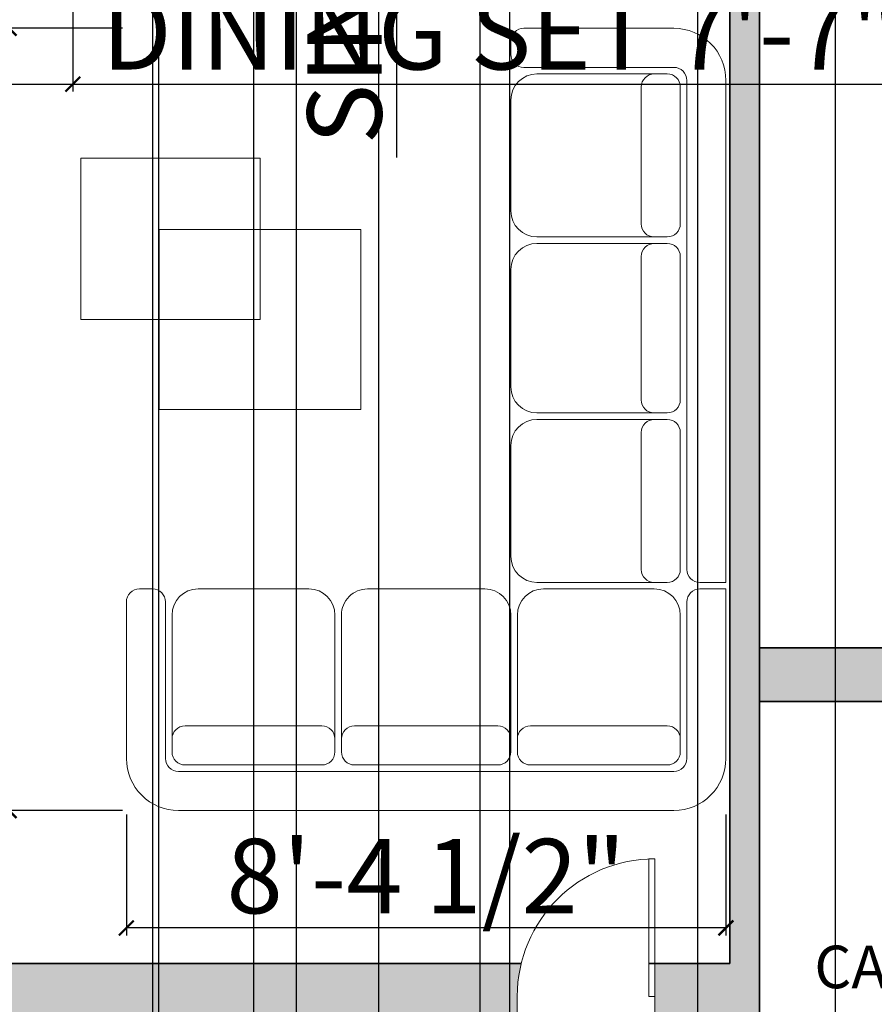
# Model space of a CAD drawing. Units: inches. Extents: x 1763 to 2368, y 1500 to 2097.
# Tile 4 of 24: x 1936 to 2079, y 1628 to 1794. Entities that reach past the tile are written whole.
import ezdxf

# ---------------------------------------------------------------- set-up
doc = ezdxf.new("R2010")
doc.units = ezdxf.units.IN
for name, color, linetype, lineweight in [('A-ANNO-DIMS', 2, 'Continuous', 18), ('A-AREA-IDEN', 7, 'Continuous', 18), ('A-DOOR', 4, 'Continuous', 18), ('A-FURN', 8, 'Continuous', 18), ('A-WALL', 7, 'Continuous', 35), ('A-WALL-PATT', 7, 'Continuous', 13)]:
    doc.layers.add(name, color=color, linetype=linetype, lineweight=lineweight)
doc.styles.get("Standard").update_dxf_attribs({"font": 'arial.ttf'})
doc.dimstyles.new('ISO-25', dxfattribs={"dimtxt": 12.5, "dimasz": 2.5, "dimexe": 1.25, "dimexo": 0.625, "dimtad": 1, "dimdec": 0, "dimlunit": 4, "dimtxsty": 'Standard', "dimblk": 'ARCHTICK', "dimcen": 2.5, "dimclrd": 3, "dimclrt": 4, "dimadec": 0, "dimazin": 0, "dimtfac": 1, "dimtdec": 0, "dimtmove": 0, "dimatfit": 3, "dimfxl": 1, "dimarcsym": 0})

# ---------------------------------------------------------------- blocks, each defined once
blk = doc.blocks.new('A$C2AFA021D')
for p, q in [((0.8, 2.3), (0.2, 2.3)), ((0.85, 2.2), (0.85, 2.25)), ((0.2, 2.15), (0.8, 2.15)), ((0.225, 2.125), (0.275, 2.125)), ((0.75, 2.125), (0.275, 2.125)), ((0, 2.1), (0, 0.2)), ((0.15, 0.2), (0.15, 2.1)), ((0.175, 1.55), (0.175, 2.075)), ((0.325, 2.075), (0.325, 1.55)), ((0.85, 1.6), (0.85, 2.025)), ((0.275, 1.5), (0.225, 1.5)), ((0.225, 1.475), (0.275, 1.475)), ((0.275, 1.5), (0.75, 1.5)), ((0.75, 1.475), (0.275, 1.475)), ((0.175, 0.875), (0.175, 1.425)), ((0.325, 1.425), (0.325, 0.875)), ((0.85, 0.925), (0.85, 1.375)), ((0.275, 0.825), (0.225, 0.825)), ((0.225, 0.8), (0.275, 0.8)), ((0.275, 0.825), (0.75, 0.825)), ((0.75, 0.8), (0.275, 0.8)), ((0.975, 0.825), (1.4, 0.825)), ((1.625, 0.825), (2.075, 0.825)), ((2.3, 0.825), (2.725, 0.825)), ((2.9, 0.825), (2.95, 0.825)), ((2.85, 0.2), (2.85, 0.775)), ((3, 0.775), (3, 0.2)), ((0.175, 0.225), (0.175, 0.75)), ((0.325, 0.75), (0.325, 0.225)), ((0.875, 0.275), (0.875, 0.725)), ((1.5, 0.725), (1.5, 0.275)), ((1.525, 0.275), (1.525, 0.725)), ((2.175, 0.725), (2.175, 0.275)), ((2.2, 0.275), (2.2, 0.725)), ((2.825, 0.725), (2.825, 0.275)), ((0.85, 0.275), (0.85, 0.7)), ((1.45, 0.325), (0.925, 0.325)), ((2.125, 0.325), (1.575, 0.325)), ((2.775, 0.325), (2.25, 0.325)), ((0.875, 0.275), (0.875, 0.225)), ((1.5, 0.225), (1.5, 0.275)), ((1.525, 0.275), (1.525, 0.225)), ((2.175, 0.225), (2.175, 0.275)), ((2.2, 0.275), (2.2, 0.225)), ((2.825, 0.225), (2.825, 0.275)), ((0.275, 0.175), (0.225, 0.175)), ((0.275, 0.175), (0.75, 0.175)), ((0.925, 0.175), (1.45, 0.175)), ((1.575, 0.175), (2.125, 0.175)), ((2.25, 0.175), (2.775, 0.175)), ((0.8, 0.15), (0.2, 0.15)), ((0.925, 0.15), (2.8, 0.15)), ((0.85, 0), (0.85, 0.1)), ((0.875, 0.1), (0.875, 0)), ((0.2, 0), (0.85, 0)), ((2.8, 0), (0.875, 0))]:
    blk.add_line(p, q)
for centre, radius, start, end in [((0.2, 2.1), 0.2, 90, 180), ((0.8, 2.25), 0.05, 0, 90), ((0.8, 2.2), 0.05, 270, 0), ((0.2, 2.1), 0.05, 90, 180), ((0.225, 2.075), 0.05, 90, 180), ((0.275, 2.075), 0.05, 0, 90), ((0.75, 2.025), 0.1, 0, 90), ((0.75, 1.6), 0.1, 270, 0), ((0.225, 1.55), 0.05, 180, 270), ((0.275, 1.55), 0.05, 270, 0), ((0.225, 1.425), 0.05, 90, 180), ((0.275, 1.425), 0.05, 0, 90), ((0.75, 1.375), 0.1, 360, 90), ((0.75, 0.925), 0.1, 270, 0), ((0.225, 0.875), 0.05, 180, 270), ((0.275, 0.875), 0.05, 270, 0), ((0.225, 0.75), 0.05, 90, 180), ((0.275, 0.75), 0.05, 0, 90), ((0.75, 0.7), 0.1, 0, 90), ((0.975, 0.725), 0.1, 90, 180), ((1.4, 0.725), 0.1, 0, 90), ((1.625, 0.725), 0.1, 90, 180), ((2.075, 0.725), 0.1, 0, 90), ((2.3, 0.725), 0.1, 90, 180), ((2.725, 0.725), 0.1, 0, 90), ((2.9, 0.775), 0.05, 90, 180), ((2.95, 0.775), 0.05, 0, 90), ((0.925, 0.275), 0.05, 90, 180), ((1.45, 0.275), 0.05, 360, 90), ((1.575, 0.275), 0.05, 90, 180), ((2.125, 0.275), 0.05, 360, 90), ((2.25, 0.275), 0.05, 90, 180), ((2.775, 0.275), 0.05, 360, 90), ((0.75, 0.275), 0.1, 270, 0), ((0.2, 0.2), 0.2, 180, 270), ((0.2, 0.2), 0.05, 180, 270), ((0.225, 0.225), 0.05, 180, 270), ((0.275, 0.225), 0.05, 270, 0), ((0.925, 0.225), 0.05, 180, 270), ((1.45, 0.225), 0.05, 270, 0), ((1.575, 0.225), 0.05, 180, 270), ((2.125, 0.225), 0.05, 270, 0), ((2.25, 0.225), 0.05, 180, 270), ((2.775, 0.225), 0.05, 270, 0), ((2.8, 0.2), 0.2, 270, 0), ((2.8, 0.2), 0.05, 270, 0), ((0.8, 0.1), 0.05, 0, 90), ((0.925, 0.1), 0.05, 90, 180)]:
    blk.add_arc(centre, radius, start, end)
blk = doc.blocks.new('*U3')
for p, q in [((0, 0), (0, -6)), ((40, 0), (40, -6))]:
    blk.add_line(p, q)
blk.add_lwpolyline([(0, 0), (0, 40), (1.75, 40), (1.75, 0)], close=True)
blk.add_arc((0, 0), 40, 0, 90)
blk = doc.blocks.new('_ArchTick')
at = {"color": 0, "linetype": 'ByBlock', "const_width": 0.15}
blk.add_lwpolyline([(-0.5, -0.5), (0.5, 0.5)], dxfattribs=at)
blk = doc.blocks.new('*D25')
at = {"layer": 'A-ANNO-DIMS', "color": 3, "lineweight": -2, "transparency": 16777216}
for p, q in [((1934.01, 1792.31), (1934.01, 1981.61)), ((1934.01, 1660.94), (1934.01, 1792.31))]:
    blk.add_line(p, q, dxfattribs=at)
at = {"layer": 'A-ANNO-DIMS', "color": 0, "lineweight": -2, "transparency": 16777216}
for p, q in [((1953.09, 1792.31), (1932.76, 1792.31)), ((1953.09, 1660.94), (1932.76, 1660.94))]:
    blk.add_line(p, q, dxfattribs=at)
at = {"layer": 'Defpoints', "color": 0, "transparency": 16777216}
for p in [(1934.01, 1792.31), (1953.72, 1792.31), (1953.72, 1660.94)]:
    blk.add_point(p, dxfattribs=at)
at = {"layer": 'A-ANNO-DIMS', "color": 3, "lineweight": -2, "transparency": 16777216, "xscale": 2.5, "yscale": 2.5, "zscale": 2.5}
for p, rotation in [((1934.01, 1792.31), 90), ((1934.01, 1660.94), 270)]:
    blk.add_blockref('_ArchTick', p, dxfattribs=dict(at, rotation=rotation))
at = {"layer": 'A-ANNO-DIMS', "color": 4, "transparency": 16777216, "insert": (1926.92, 1888.21), "char_height": 12.5, "attachment_point": 5, "rotation": 90}
blk.add_mtext('SECTIONAL 10\'-11 1/2"', dxfattribs=at)
blk = doc.blocks.new('*D26')
at = {"layer": 'A-ANNO-DIMS', "color": 0, "lineweight": -2, "transparency": 16777216}
for p, q in [((1953.72, 1660.31), (1953.72, 1639.98)), ((2054.44, 1660.31), (2054.44, 1639.98))]:
    blk.add_line(p, q, dxfattribs=at)
at = {"layer": 'A-ANNO-DIMS', "color": 3, "lineweight": -2, "transparency": 16777216}
blk.add_line((2054.44, 1641.23), (1953.72, 1641.23), dxfattribs=at)
at = {"layer": 'Defpoints', "color": 0, "transparency": 16777216}
for p in [(1953.72, 1660.94), (2054.44, 1660.94), (1953.72, 1641.23)]:
    blk.add_point(p, dxfattribs=at)
at = {"layer": 'A-ANNO-DIMS', "color": 3, "lineweight": -2, "transparency": 16777216, "xscale": 2.5, "yscale": 2.5, "zscale": 2.5, "rotation": 180}
blk.add_blockref('_ArchTick', (1953.72, 1641.23), dxfattribs=at)
at = {"layer": 'A-ANNO-DIMS', "color": 3, "lineweight": -2, "transparency": 16777216, "xscale": 2.5, "yscale": 2.5, "zscale": 2.5}
blk.add_blockref('_ArchTick', (2054.44, 1641.23), dxfattribs=at)
at = {"layer": 'A-ANNO-DIMS', "color": 4, "transparency": 16777216, "insert": (2004.08, 1648.32), "char_height": 12.5, "attachment_point": 5}
blk.add_mtext('8\'-4 1/2"', dxfattribs=at)
blk = doc.blocks.new('*D27')
at = {"layer": 'A-ANNO-DIMS', "color": 0, "lineweight": -2, "transparency": 16777216}
for p, q in [((1853.71, 1795.96), (1853.71, 1781.68)), ((1944.71, 1795.96), (1944.71, 1781.68))]:
    blk.add_line(p, q, dxfattribs=at)
at = {"layer": 'A-ANNO-DIMS', "color": 3, "lineweight": -2, "transparency": 16777216}
for p, q in [((1853.71, 1782.93), (1944.71, 1782.93)), ((1944.71, 1782.93), (2085.85, 1782.93))]:
    blk.add_line(p, q, dxfattribs=at)
at = {"layer": 'Defpoints', "color": 0, "transparency": 16777216}
for p in [(1853.71, 1796.58), (1944.71, 1796.58), (1944.71, 1782.93)]:
    blk.add_point(p, dxfattribs=at)
at = {"layer": 'A-ANNO-DIMS', "color": 3, "lineweight": -2, "transparency": 16777216, "xscale": 2.5, "yscale": 2.5, "zscale": 2.5, "rotation": 180}
blk.add_blockref('_ArchTick', (1853.71, 1782.93), dxfattribs=at)
at = {"layer": 'A-ANNO-DIMS', "color": 3, "lineweight": -2, "transparency": 16777216, "xscale": 2.5, "yscale": 2.5, "zscale": 2.5}
blk.add_blockref('_ArchTick', (1944.71, 1782.93), dxfattribs=at)
at = {"layer": 'A-ANNO-DIMS', "color": 4, "transparency": 16777216, "insert": (2016.53, 1790.02), "char_height": 12.5, "attachment_point": 5}
blk.add_mtext('DINING SET 7\'-7"', dxfattribs=at)
blk = doc.blocks.new('*D33')
at = {"layer": 'A-ANNO-DIMS', "color": 0, "lineweight": -2, "transparency": 16777216}
for p, q in [((2001.02, 1913.28), (1997.82, 1913.28)), ((2001.02, 1896.11), (1997.82, 1896.11))]:
    blk.add_line(p, q, dxfattribs=at)
at = {"layer": 'A-ANNO-DIMS', "color": 3, "lineweight": -2, "transparency": 16777216}
for p, q in [((1999.07, 1913.28), (1999.07, 1896.11)), ((1999.07, 1896.11), (1999.07, 1770.61))]:
    blk.add_line(p, q, dxfattribs=at)
at = {"layer": 'Defpoints', "color": 0, "transparency": 16777216}
for p in [(2001.64, 1913.28), (1999.07, 1896.11), (2001.64, 1896.11)]:
    blk.add_point(p, dxfattribs=at)
at = {"layer": 'A-ANNO-DIMS', "color": 3, "lineweight": -2, "transparency": 16777216, "xscale": 2.5, "yscale": 2.5, "zscale": 2.5}
for p, rotation in [((1999.07, 1913.28), 90), ((1999.07, 1896.11), 270)]:
    blk.add_blockref('_ArchTick', p, dxfattribs=dict(at, rotation=rotation))
at = {"layer": 'A-ANNO-DIMS', "color": 4, "transparency": 16777216, "insert": (1991.98, 1832.11), "char_height": 12.5, "attachment_point": 5, "rotation": 90}
blk.add_mtext('SINK 1\'-5" TYP.', dxfattribs=at)
blk = doc.blocks.new('*D58')
at = {"layer": 'A-ANNO-DIMS', "color": 0, "lineweight": -2, "transparency": 16777216}
for p, q in [((1871.68, 1635.9), (1871.68, 2072.02)), ((1927.07, 1635.9), (1927.07, 2072.02))]:
    blk.add_line(p, q, dxfattribs=at)
at = {"layer": 'A-ANNO-DIMS', "color": 3, "lineweight": -2, "transparency": 16777216}
for p, q in [((1871.68, 2070.77), (1927.07, 2070.77)), ((1927.07, 2070.77), (1993.68, 2070.77))]:
    blk.add_line(p, q, dxfattribs=at)
at = {"layer": 'Defpoints', "color": 0, "transparency": 16777216}
for p in [(1927.07, 2070.77), (1871.68, 1635.27), (1927.07, 1635.27)]:
    blk.add_point(p, dxfattribs=at)
at = {"layer": 'A-ANNO-DIMS', "color": 3, "lineweight": -2, "transparency": 16777216, "xscale": 2.5, "yscale": 2.5, "zscale": 2.5, "rotation": 180}
blk.add_blockref('_ArchTick', (1871.68, 2070.77), dxfattribs=at)
at = {"layer": 'A-ANNO-DIMS', "color": 3, "lineweight": -2, "transparency": 16777216, "xscale": 2.5, "yscale": 2.5, "zscale": 2.5}
blk.add_blockref('_ArchTick', (1927.07, 2070.77), dxfattribs=at)
at = {"layer": 'A-ANNO-DIMS', "color": 4, "transparency": 16777216, "insert": (1961.63, 2077.86), "char_height": 12.5, "attachment_point": 5}
blk.add_mtext('4\'-7 1/2"', dxfattribs=at)
blk = doc.blocks.new('*D60')
at = {"layer": 'A-ANNO-DIMS', "color": 0, "lineweight": -2, "transparency": 16777216}
for p, q in [((2060.09, 1678.65), (2060.09, 1509.91)), ((2100.58, 1678.65), (2100.58, 1509.91))]:
    blk.add_line(p, q, dxfattribs=at)
at = {"layer": 'A-ANNO-DIMS', "color": 3, "lineweight": -2, "transparency": 16777216}
for p, q in [((2060.09, 1511.16), (2100.58, 1511.16)), ((2100.58, 1511.16), (2166.67, 1511.16))]:
    blk.add_line(p, q, dxfattribs=at)
at = {"layer": 'Defpoints', "color": 0, "transparency": 16777216}
for p in [(2060.09, 1679.27), (2100.58, 1679.27), (2100.58, 1511.16)]:
    blk.add_point(p, dxfattribs=at)
at = {"layer": 'A-ANNO-DIMS', "color": 3, "lineweight": -2, "transparency": 16777216, "xscale": 2.5, "yscale": 2.5, "zscale": 2.5, "rotation": 180}
blk.add_blockref('_ArchTick', (2060.09, 1511.16), dxfattribs=at)
at = {"layer": 'A-ANNO-DIMS', "color": 3, "lineweight": -2, "transparency": 16777216, "xscale": 2.5, "yscale": 2.5, "zscale": 2.5}
blk.add_blockref('_ArchTick', (2100.58, 1511.16), dxfattribs=at)
at = {"layer": 'A-ANNO-DIMS', "color": 4, "transparency": 16777216, "insert": (2134.88, 1518.25), "char_height": 12.5, "attachment_point": 5}
blk.add_mtext('3\'-4 1/2"', dxfattribs=at)
blk = doc.blocks.new('*D68')
at = {"layer": 'A-ANNO-DIMS', "color": 0, "lineweight": -2, "transparency": 16777216}
for p, q in [((1895.59, 1879.65), (1895.59, 1509.91)), ((1932.01, 1879.65), (1932.01, 1509.91))]:
    blk.add_line(p, q, dxfattribs=at)
at = {"layer": 'A-ANNO-DIMS', "color": 3, "lineweight": -2, "transparency": 16777216}
for p, q in [((1895.59, 1511.16), (1932.01, 1511.16)), ((1932.01, 1511.16), (1998.11, 1511.16))]:
    blk.add_line(p, q, dxfattribs=at)
at = {"layer": 'Defpoints', "color": 0, "transparency": 16777216}
for p in [(1895.59, 1880.27), (1932.01, 1880.27), (1932.01, 1511.16)]:
    blk.add_point(p, dxfattribs=at)
at = {"layer": 'A-ANNO-DIMS', "color": 3, "lineweight": -2, "transparency": 16777216, "xscale": 2.5, "yscale": 2.5, "zscale": 2.5, "rotation": 180}
blk.add_blockref('_ArchTick', (1895.59, 1511.16), dxfattribs=at)
at = {"layer": 'A-ANNO-DIMS', "color": 3, "lineweight": -2, "transparency": 16777216, "xscale": 2.5, "yscale": 2.5, "zscale": 2.5}
blk.add_blockref('_ArchTick', (1932.01, 1511.16), dxfattribs=at)
at = {"layer": 'A-ANNO-DIMS', "color": 4, "transparency": 16777216, "insert": (1966.31, 1518.25), "char_height": 12.5, "attachment_point": 5}
blk.add_mtext('3\'-0 1/2"', dxfattribs=at)
blk = doc.blocks.new('*D69')
at = {"layer": 'A-ANNO-DIMS', "color": 0, "lineweight": -2, "transparency": 16777216}
for p, q in [((1838.09, 1879.65), (1838.09, 1509.91)), ((1895.59, 1879.65), (1895.59, 1509.91))]:
    blk.add_line(p, q, dxfattribs=at)
at = {"layer": 'A-ANNO-DIMS', "color": 3, "lineweight": -2, "transparency": 16777216}
for p, q in [((1838.09, 1511.16), (1895.59, 1511.16)), ((1895.59, 1511.16), (1962.2, 1511.16))]:
    blk.add_line(p, q, dxfattribs=at)
at = {"layer": 'Defpoints', "color": 0, "transparency": 16777216}
for p in [(1838.09, 1880.27), (1895.59, 1880.27), (1895.59, 1511.16)]:
    blk.add_point(p, dxfattribs=at)
at = {"layer": 'A-ANNO-DIMS', "color": 3, "lineweight": -2, "transparency": 16777216, "xscale": 2.5, "yscale": 2.5, "zscale": 2.5, "rotation": 180}
blk.add_blockref('_ArchTick', (1838.09, 1511.16), dxfattribs=at)
at = {"layer": 'A-ANNO-DIMS', "color": 3, "lineweight": -2, "transparency": 16777216, "xscale": 2.5, "yscale": 2.5, "zscale": 2.5}
blk.add_blockref('_ArchTick', (1895.59, 1511.16), dxfattribs=at)
at = {"layer": 'A-ANNO-DIMS', "color": 4, "transparency": 16777216, "insert": (1930.15, 1518.24), "char_height": 12.5, "attachment_point": 5}
blk.add_mtext('4\'-9 1/2"', dxfattribs=at)
blk = doc.blocks.new('*D70')
at = {"layer": 'A-ANNO-DIMS', "color": 0, "lineweight": -2, "transparency": 16777216}
for p, q in [((1959.13, 1879.65), (1959.13, 1509.91)), ((1982.23, 1879.65), (1982.23, 1509.91))]:
    blk.add_line(p, q, dxfattribs=at)
at = {"layer": 'A-ANNO-DIMS', "color": 3, "lineweight": -2, "transparency": 16777216}
for p, q in [((1959.13, 1511.16), (1982.23, 1511.16)), ((1982.23, 1511.16), (2027.75, 1511.16))]:
    blk.add_line(p, q, dxfattribs=at)
at = {"layer": 'Defpoints', "color": 0, "transparency": 16777216}
for p in [(1959.13, 1880.27), (1982.23, 1880.27), (1982.23, 1511.16)]:
    blk.add_point(p, dxfattribs=at)
at = {"layer": 'A-ANNO-DIMS', "color": 3, "lineweight": -2, "transparency": 16777216, "xscale": 2.5, "yscale": 2.5, "zscale": 2.5, "rotation": 180}
blk.add_blockref('_ArchTick', (1959.13, 1511.16), dxfattribs=at)
at = {"layer": 'A-ANNO-DIMS', "color": 3, "lineweight": -2, "transparency": 16777216, "xscale": 2.5, "yscale": 2.5, "zscale": 2.5}
blk.add_blockref('_ArchTick', (1982.23, 1511.16), dxfattribs=at)
at = {"layer": 'A-ANNO-DIMS', "color": 4, "transparency": 16777216, "insert": (2006.24, 1518.06), "char_height": 12.5, "attachment_point": 5}
blk.add_mtext('1\'-11"', dxfattribs=at)
blk = doc.blocks.new('*D71')
at = {"layer": 'A-ANNO-DIMS', "color": 0, "lineweight": -2, "transparency": 16777216}
for p, q in [((2049.69, 1879.65), (2049.69, 1509.91)), ((2072.78, 1879.65), (2072.78, 1509.91))]:
    blk.add_line(p, q, dxfattribs=at)
at = {"layer": 'A-ANNO-DIMS', "color": 3, "lineweight": -2, "transparency": 16777216}
for p, q in [((2049.69, 1511.16), (2072.78, 1511.16)), ((2072.78, 1511.16), (2118.3, 1511.16))]:
    blk.add_line(p, q, dxfattribs=at)
at = {"layer": 'Defpoints', "color": 0, "transparency": 16777216}
for p in [(2049.69, 1880.27), (2072.78, 1880.27), (2072.78, 1511.16)]:
    blk.add_point(p, dxfattribs=at)
at = {"layer": 'A-ANNO-DIMS', "color": 3, "lineweight": -2, "transparency": 16777216, "xscale": 2.5, "yscale": 2.5, "zscale": 2.5, "rotation": 180}
blk.add_blockref('_ArchTick', (2049.69, 1511.16), dxfattribs=at)
at = {"layer": 'A-ANNO-DIMS', "color": 3, "lineweight": -2, "transparency": 16777216, "xscale": 2.5, "yscale": 2.5, "zscale": 2.5}
blk.add_blockref('_ArchTick', (2072.78, 1511.16), dxfattribs=at)
at = {"layer": 'A-ANNO-DIMS', "color": 4, "transparency": 16777216, "insert": (2096.79, 1518.06), "char_height": 12.5, "attachment_point": 5}
blk.add_mtext('1\'-11"', dxfattribs=at)
blk = doc.blocks.new('*D77')
at = {"layer": 'A-ANNO-DIMS', "color": 0, "lineweight": -2, "transparency": 16777216}
for p, q in [((1975.09, 1972.65), (1975.09, 1509.91)), ((1996.09, 1972.65), (1996.09, 1509.91))]:
    blk.add_line(p, q, dxfattribs=at)
at = {"layer": 'A-ANNO-DIMS', "color": 3, "lineweight": -2, "transparency": 16777216}
for p, q in [((1975.09, 1511.16), (1996.09, 1511.16)), ((1996.09, 1511.16), (2031.89, 1511.16))]:
    blk.add_line(p, q, dxfattribs=at)
at = {"layer": 'Defpoints', "color": 0, "transparency": 16777216}
for p in [(1975.09, 1973.27), (1996.09, 1973.27), (1996.09, 1511.16)]:
    blk.add_point(p, dxfattribs=at)
at = {"layer": 'A-ANNO-DIMS', "color": 3, "lineweight": -2, "transparency": 16777216, "xscale": 2.5, "yscale": 2.5, "zscale": 2.5, "rotation": 180}
blk.add_blockref('_ArchTick', (1975.09, 1511.16), dxfattribs=at)
at = {"layer": 'A-ANNO-DIMS', "color": 3, "lineweight": -2, "transparency": 16777216, "xscale": 2.5, "yscale": 2.5, "zscale": 2.5}
blk.add_blockref('_ArchTick', (1996.09, 1511.16), dxfattribs=at)
at = {"layer": 'A-ANNO-DIMS', "color": 4, "transparency": 16777216, "insert": (2015.24, 1518.16), "char_height": 12.5, "attachment_point": 5}
blk.add_mtext('1\'-9"', dxfattribs=at)
blk = doc.blocks.new('*D86')
at = {"layer": 'A-ANNO-DIMS', "color": 0, "lineweight": -2, "transparency": 16777216}
for p, q in [((2013.09, 1884.65), (2013.09, 1509.91)), ((2018.09, 1884.65), (2018.09, 1509.91))]:
    blk.add_line(p, q, dxfattribs=at)
at = {"layer": 'A-ANNO-DIMS', "color": 3, "lineweight": -2, "transparency": 16777216}
for p, q in [((2013.09, 1511.16), (2018.09, 1511.16)), ((2018.09, 1511.16), (2055.07, 1511.16))]:
    blk.add_line(p, q, dxfattribs=at)
at = {"layer": 'Defpoints', "color": 0, "transparency": 16777216}
for p in [(2013.09, 1885.27), (2018.09, 1885.27), (2018.09, 1511.16)]:
    blk.add_point(p, dxfattribs=at)
at = {"layer": 'A-ANNO-DIMS', "color": 3, "lineweight": -2, "transparency": 16777216, "xscale": 2.5, "yscale": 2.5, "zscale": 2.5, "rotation": 180}
blk.add_blockref('_ArchTick', (2013.09, 1511.16), dxfattribs=at)
at = {"layer": 'A-ANNO-DIMS', "color": 3, "lineweight": -2, "transparency": 16777216, "xscale": 2.5, "yscale": 2.5, "zscale": 2.5}
blk.add_blockref('_ArchTick', (2018.09, 1511.16), dxfattribs=at)
at = {"layer": 'A-ANNO-DIMS', "color": 4, "transparency": 16777216, "insert": (2037.83, 1518.16), "char_height": 12.5, "attachment_point": 5}
blk.add_mtext('0\'-5"', dxfattribs=at)
blk = doc.blocks.new('*D87')
at = {"layer": 'A-ANNO-DIMS', "color": 0, "lineweight": -2, "transparency": 16777216}
for p, q in [((1958.09, 1980.65), (1958.09, 1509.91)), ((1975.09, 1980.65), (1975.09, 1509.91))]:
    blk.add_line(p, q, dxfattribs=at)
at = {"layer": 'A-ANNO-DIMS', "color": 3, "lineweight": -2, "transparency": 16777216}
for p, q in [((1958.09, 1511.16), (1975.09, 1511.16)), ((1975.09, 1511.16), (2010.89, 1511.16))]:
    blk.add_line(p, q, dxfattribs=at)
at = {"layer": 'Defpoints', "color": 0, "transparency": 16777216}
for p in [(1958.09, 1981.27), (1975.09, 1981.27), (1975.09, 1511.16)]:
    blk.add_point(p, dxfattribs=at)
at = {"layer": 'A-ANNO-DIMS', "color": 3, "lineweight": -2, "transparency": 16777216, "xscale": 2.5, "yscale": 2.5, "zscale": 2.5, "rotation": 180}
blk.add_blockref('_ArchTick', (1958.09, 1511.16), dxfattribs=at)
at = {"layer": 'A-ANNO-DIMS', "color": 3, "lineweight": -2, "transparency": 16777216, "xscale": 2.5, "yscale": 2.5, "zscale": 2.5}
blk.add_blockref('_ArchTick', (1975.09, 1511.16), dxfattribs=at)
at = {"layer": 'A-ANNO-DIMS', "color": 4, "transparency": 16777216, "insert": (1994.24, 1518.16), "char_height": 12.5, "attachment_point": 5}
blk.add_mtext('1\'-5"', dxfattribs=at)

msp = doc.modelspace()

# ---------------------------------------------------------------- hatches: boundary and pattern name
at = {"layer": 'A-WALL-PATT'}
h = msp.add_hatch(color=256, dxfattribs=at)
h.dxf.hatch_style = 1
h.paths.add_polyline_path([(1838.09, 2034.27), (1838.09, 2043.27), (1829.09, 2043.27), (1829.09, 1953.39), (1838.09, 1953.39)])
h.paths.add_polyline_path([(1838.09, 1913.1), (1829.09, 1913.1), (1829.09, 1862.2), (1838.09, 1862.2)])
h.paths.add_polyline_path([(1838.09, 1825.59), (1829.09, 1825.59), (1829.09, 1738.64), (1838.09, 1738.64)])
h.paths.add_polyline_path([(1895.59, 1885.27), (1838.09, 1885.27), (1838.09, 1880.27), (1895.59, 1880.27)])
h.paths.add_polyline_path([(1857.39, 1784.27), (1838.09, 1784.27), (1838.09, 1779.27), (1857.39, 1779.27)])
h.paths.add_polyline_path([(1958.09, 1981.27), (1971.46, 1981.27), (1971.46, 1986.27), (1968.57, 1986.27), (1958.09, 1986.27), (1953.09, 1986.27), (1927.39, 1986.27), (1927.39, 1981.27), (1953.09, 1981.27), (1953.09, 1885.27), (1932.01, 1885.27), (1932.01, 1880.27), (1959.13, 1880.27), (1959.13, 1883.74), (1959.13, 1885.27), (1958.09, 1885.27)])
h.paths.add_polyline_path([(2018.09, 1981.27), (2031.02, 1981.27), (2031.02, 1986.27), (2018.09, 1986.27), (2013.09, 1986.27), (2001.23, 1986.27), (2001.23, 1981.27), (2013.09, 1981.27), (2013.09, 1885.27), (1982.18, 1885.27, -0.016629), (1982.23, 1883.74), (1982.23, 1880.27), (2049.69, 1880.27), (2049.69, 1883.74, -0.016629), (2049.74, 1885.27), (2018.09, 1885.27)])
h.paths.add_polyline_path([(2083.09, 1981.27), (2120.61, 1981.27), (2120.61, 1986.27), (2083.09, 1986.27), (2078.09, 1986.27), (2063.14, 1986.27), (2063.14, 1981.27), (2078.09, 1981.27), (2078.09, 1885.27), (2072.78, 1885.27), (2072.78, 1883.74), (2072.78, 1880.27), (2078.09, 1880.27), (2078.09, 1866.87), (2081.56, 1866.87, -0.016629), (2083.09, 1866.82)])
h.paths.add_polyline_path([(1871.68, 1635.27), (1838.09, 1635.27), (1838.09, 1626.27), (1871.68, 1626.27)], flags=17)
h.paths.add_polyline_path([(2100.58, 1688.27), (2060.09, 1688.27), (2060.09, 1679.27), (2100.58, 1679.27)], flags=17)
h.paths.add_polyline_path([(2180.09, 1688.27), (2148.74, 1688.27), (2148.74, 1679.27), (2180.09, 1679.27)], flags=17)
h.paths.add_polyline_path([(2189.09, 1746.22), (2180.09, 1746.22), (2180.09, 1743.42), (2180.12, 1743.42), (2180.12, 1726.72), (2180.09, 1572.27), (2034.91, 1572.27), (2034.91, 1565.6), (2034.91, 1563.27), (2189.09, 1563.27)])
h.paths.add_polyline_path([(2060.09, 1802.35, -0.016629), (2058.56, 1802.3), (2055.09, 1802.3), (2055.09, 1635.27), (2042.48, 1635.27), (2042.48, 1629.74), (2042.48, 1626.27), (2055.09, 1626.27), (2055.09, 1599.27), (2040.27, 1599.27), (2040.27, 1590.27), (2060.09, 1590.27)])
h.paths.add_polyline_path([(2019.39, 1629.74, -0.060569), (2020.06, 1635.27), (1995.09, 1635.27), (1990.09, 1635.27), (1927.07, 1635.27), (1927.07, 1626.27), (1990.09, 1626.27), (1990.09, 1590.27), (1995.09, 1590.27), (2005.2, 1590.27), (2005.2, 1599.27), (1995.09, 1599.27), (1995.09, 1626.27), (2019.39, 1626.27)])
edge = h.paths.add_edge_path()
edge.add_line((2180.09, 1837.27), (2167.2, 1837.27))
edge.add_spline(control_points=[(2167.2, 1837.27), (2167.19, 1837.27), (2167.18, 1837.27), (2167.18, 1837.27)], knot_values=[168.955493, 168.955493, 168.955493, 168.955493, 169.065871, 169.065871, 169.065871, 169.065871], degree=3, periodic=0)
edge.add_spline(control_points=[(2167.18, 1837.27), (2166.56, 1837.38), (2166.33, 1846.16), (2165.71, 1846.24)], knot_values=[159.864705, 159.864705, 159.864705, 159.864705, 168.955493, 168.955493, 168.955493, 168.955493], degree=3, periodic=0)
edge.add_line((2167.12, 1837.27), (2163.16, 1837.27))
edge.add_spline(control_points=[(2163.16, 1837.27), (2163.16, 1837.27), (2163.16, 1837.27), (2163.15, 1837.27)], knot_values=[150.537172, 150.537172, 150.537172, 150.537172, 150.553797, 150.553797, 150.553797, 150.553797], degree=3, periodic=0)
edge.add_spline(control_points=[(2163.15, 1837.27), (2162.29, 1837.29), (2161.59, 1846.23), (2160.88, 1846.24)], knot_values=[141.293426, 141.293426, 141.293426, 141.293426, 150.537172, 150.537172, 150.537172, 150.537172], degree=3, periodic=0)
edge.add_line((2163.08, 1837.27), (2158.7, 1837.27))
edge.add_spline(control_points=[(2158.7, 1837.27), (2158.7, 1837.27), (2158.7, 1837.27), (2158.7, 1837.27)], knot_values=[132.033544, 132.033544, 132.033544, 132.033544, 132.049151, 132.049151, 132.049151, 132.049151], degree=3, periodic=0)
edge.add_spline(control_points=[(2158.7, 1837.27), (2157.97, 1837.29), (2157.26, 1846.23), (2156.39, 1846.24)], knot_values=[122.786021, 122.786021, 122.786021, 122.786021, 132.033544, 132.033544, 132.033544, 132.033544], degree=3, periodic=0)
edge.add_line((2158.63, 1837.27), (2153.84, 1837.27))
edge.add_spline(control_points=[(2153.84, 1837.27), (2153.83, 1837.27), (2153.82, 1837.27), (2153.82, 1837.27)], knot_values=[113.451585, 113.451585, 113.451585, 113.451585, 113.562103, 113.562103, 113.562103, 113.562103], degree=3, periodic=0)
edge.add_spline(control_points=[(2153.82, 1837.27), (2153.17, 1837.38), (2152.88, 1846.19), (2152.4, 1846.24)], knot_values=[0, 0, 0, 0, 9.081854, 9.081854, 9.081854, 9.081854], degree=3, periodic=0)
edge.add_line((2153.76, 1837.27), (2150.39, 1837.27))
edge.add_spline(control_points=[(2150.39, 1837.27), (2150.38, 1837.27), (2150.37, 1837.27), (2150.36, 1837.27)], knot_values=[95.069382, 95.069382, 95.069382, 95.069382, 95.17519, 95.17519, 95.17519, 95.17519], degree=3, periodic=0)
edge.add_spline(control_points=[(2150.36, 1837.27), (2149.49, 1837.37), (2148.42, 1846.19), (2147.59, 1846.24)], knot_values=[85.824599, 85.824599, 85.824599, 85.824599, 95.069382, 95.069382, 95.069382, 95.069382], degree=3, periodic=0)
edge.add_line((2150.29, 1837.27), (2145.43, 1837.27))
edge.add_spline(control_points=[(2145.43, 1837.27), (2145.43, 1837.27), (2145.42, 1837.27), (2145.42, 1837.27)], knot_values=[76.505559, 76.505559, 76.505559, 76.505559, 76.547811, 76.547811, 76.547811, 76.547811], degree=3, periodic=0)
edge.add_spline(control_points=[(2145.42, 1837.27), (2144.68, 1837.31), (2143.8, 1846.19), (2142.95, 1846.24)], knot_values=[67.23945, 67.23945, 67.23945, 67.23945, 76.505559, 76.505559, 76.505559, 76.505559], degree=3, periodic=0)
edge.add_line((2145.35, 1837.27), (2134.57, 1837.27))
edge.add_spline(control_points=[(2134.57, 1837.27), (2134.57, 1837.27), (2134.56, 1837.27), (2134.56, 1837.27)], knot_values=[39.001463, 39.001463, 39.001463, 39.001463, 39.045107, 39.045107, 39.045107, 39.045107], degree=3, periodic=0)
edge.add_spline(control_points=[(2134.56, 1837.27), (2133.87, 1837.31), (2133.4, 1845.85), (2132.33, 1846.24)], knot_values=[29.79778, 29.79778, 29.79778, 29.79778, 39.001463, 39.001463, 39.001463, 39.001463], degree=3, periodic=0)
edge.add_line((2134.5, 1837.27), (2128.08, 1837.27))
edge.add_spline(control_points=[(2128.08, 1837.27), (2128.03, 1837.26), (2127.98, 1837.26), (2127.93, 1837.27)], knot_values=[19.482067, 19.482067, 19.482067, 19.482067, 19.869396, 19.869396, 19.869396, 19.869396], degree=3, periodic=0)
edge.add_spline(control_points=[(2125.01, 1846.24), (2126.16, 1844.66), (2126.82, 1837.57), (2127.93, 1837.27)], knot_values=[10.389805, 10.389805, 10.389805, 10.389805, 19.482067, 19.482067, 19.482067, 19.482067], degree=3, periodic=0)
edge.add_line((2127.93, 1837.27), (2083.09, 1837.27))
edge.add_line((2083.09, 1837.27), (2083.09, 1843.77))
edge.add_line((2083.09, 1843.77), (2081.56, 1843.77))
edge.add_line((2081.56, 1843.77), (2078.09, 1843.77))
edge.add_line((2078.09, 1843.77), (2078.09, 1837.27))
edge.add_line((2078.09, 1837.27), (2055.09, 1837.27))
edge.add_line((2055.09, 1837.27), (2055.09, 1825.4))
edge.add_line((2055.09, 1825.4), (2058.56, 1825.4))
edge.add_line((2058.56, 1825.4), (2060.09, 1825.4))
edge.add_line((2060.09, 1825.4), (2060.09, 1832.27))
edge.add_line((2060.09, 1832.27), (2122.44, 1832.27))
edge.add_spline(control_points=[(2122.44, 1832.27), (2122.73, 1832.58), (2123.01, 1832.62), (2123.28, 1832.27)], knot_values=[5.972033, 5.972033, 5.972033, 5.972033, 8.057258, 8.057258, 8.057258, 8.057258], degree=3, periodic=0)
edge.add_line((2123.28, 1832.27), (2137.95, 1832.27))
edge.add_spline(control_points=[(2137.95, 1832.27), (2137.96, 1832.27), (2137.97, 1832.27), (2137.98, 1832.27)], knot_values=[53.926862, 53.926862, 53.926862, 53.926862, 54.030075, 54.030075, 54.030075, 54.030075], degree=3, periodic=0)
edge.add_spline(control_points=[(2139.72, 1825.02), (2139.28, 1825.06), (2138.67, 1832.18), (2137.98, 1832.27)], knot_values=[54.030075, 54.030075, 54.030075, 54.030075, 61.445194, 61.445194, 61.445194, 61.445194], degree=3, periodic=0)
edge.add_line((2138.05, 1832.27), (2140.96, 1832.27))
edge.add_spline(control_points=[(2140.96, 1832.27), (2140.97, 1832.27), (2140.98, 1832.27), (2140.99, 1832.27)], knot_values=[68.854182, 68.854182, 68.854182, 68.854182, 68.971237, 68.971237, 68.971237, 68.971237], degree=3, periodic=0)
edge.add_spline(control_points=[(2143.19, 1825.02), (2142.44, 1825.07), (2141.56, 1832.16), (2140.99, 1832.27)], knot_values=[68.971237, 68.971237, 68.971237, 68.971237, 76.444911, 76.444911, 76.444911, 76.444911], degree=3, periodic=0)
edge.add_line((2141.04, 1832.27), (2145.43, 1832.27))
edge.add_spline(control_points=[(2145.43, 1832.27), (2145.44, 1832.27), (2145.45, 1832.27), (2145.46, 1832.27)], knot_values=[84.039047, 84.039047, 84.039047, 84.039047, 84.124041, 84.124041, 84.124041, 84.124041], degree=3, periodic=0)
edge.add_spline(control_points=[(2148.11, 1825.02), (2147.34, 1825.02), (2146.3, 1832.19), (2145.46, 1832.27)], knot_values=[84.124041, 84.124041, 84.124041, 84.124041, 91.773891, 91.773891, 91.773891, 91.773891], degree=3, periodic=0)
edge.add_line((2145.54, 1832.27), (2150.39, 1832.27))
edge.add_spline(control_points=[(2150.39, 1832.27), (2150.42, 1832.28), (2150.45, 1832.28), (2150.47, 1832.27)], knot_values=[99.381577, 99.381577, 99.381577, 99.381577, 99.573457, 99.573457, 99.573457, 99.573457], degree=3, periodic=0)
edge.add_spline(control_points=[(2153.97, 1825.02), (2153.09, 1825.28), (2151.53, 1832.1), (2150.47, 1832.27)], knot_values=[99.573457, 99.573457, 99.573457, 99.573457, 107.218357, 107.218357, 107.218357, 107.218357], degree=3, periodic=0)
edge.add_line((2150.57, 1832.27), (2155.6, 1832.27))
edge.add_spline(control_points=[(2155.6, 1832.27), (2155.6, 1832.27), (2155.61, 1832.27), (2155.62, 1832.27)], knot_values=[114.933058, 114.933058, 114.933058, 114.933058, 115.013624, 115.013624, 115.013624, 115.013624], degree=3, periodic=0)
edge.add_spline(control_points=[(2158.28, 1825.02), (2157.4, 1825.07), (2156.25, 1832.2), (2155.62, 1832.27)], knot_values=[115.013624, 115.013624, 115.013624, 115.013624, 122.616269, 122.616269, 122.616269, 122.616269], degree=3, periodic=0)
edge.add_line((2155.68, 1832.27), (2165.19, 1832.27))
edge.add_spline(control_points=[(2165.19, 1832.27), (2165.2, 1832.27), (2165.2, 1832.27), (2165.2, 1832.27)], knot_values=[145.488477, 145.488477, 145.488477, 145.488477, 145.516379, 145.516379, 145.516379, 145.516379], degree=3, periodic=0)
edge.add_spline(control_points=[(2167.45, 1825.02), (2166.96, 1825.02), (2166.06, 1832.25), (2165.2, 1832.27)], knot_values=[145.516379, 145.516379, 145.516379, 145.516379, 153.105469, 153.105469, 153.105469, 153.105469], degree=3, periodic=0)
edge.add_line((2165.29, 1832.27), (2168.93, 1832.27))
edge.add_spline(control_points=[(2168.93, 1832.27), (2168.98, 1832.29), (2169.04, 1832.29), (2169.1, 1832.27)], knot_values=[160.517439, 160.517439, 160.517439, 160.517439, 160.939723, 160.939723, 160.939723, 160.939723], degree=3, periodic=0)
edge.add_spline(control_points=[(2171.09, 1828.64), (2170.35, 1830.37), (2169.62, 1832.09), (2169.1, 1832.27)], knot_values=[160.939723, 160.939723, 160.939723, 160.939723, 164.738835, 164.738835, 164.738835, 164.738835], degree=3, periodic=0)
edge.add_line((2169.1, 1832.27), (2180.09, 1832.27))
edge.add_line((2180.09, 1832.27), (2180.09, 1837.27))
h.paths.add_polyline_path([(2189.09, 1885.52), (2180.09, 1885.52), (2180.09, 1813.32), (2180.12, 1813.32), (2180.12, 1796.62), (2180.12, 1795.26), (2189.09, 1795.26)])
h.paths.add_polyline_path([(2180.09, 1986.27), (2166.28, 1986.27), (2166.28, 1981.27), (2180.09, 1981.27)])
h.paths.add_polyline_path([(2189.09, 2043.27), (2180.09, 2043.27), (2180.09, 2034.27), (2180.09, 1934.11), (2189.09, 1934.11)])
h.paths.add_polyline_path([(1838.09, 1681.59), (1829.09, 1681.59), (1829.09, 1563.27), (2003.86, 1563.27), (2003.86, 1565.6), (2003.86, 1572.27), (1838.09, 1572.27)])

# ---------------------------------------------------------------- linework, layer by layer
at = {"layer": 'A-FURN'}
for points in [[(1976.19, 1743.4), (1946.09, 1743.4), (1946.09, 1770.53), (1976.19, 1770.53)], [(1959.25, 1758.52), (1993.13, 1758.52), (1993.13, 1728.28), (1959.25, 1728.28)]]:
    msp.add_lwpolyline(points, close=True, dxfattribs=at)
at = {"layer": 'A-WALL'}
for p, q in [((2055.09, 1802.3), (2055.09, 1635.27)), ((2060.09, 1802.35), (2060.09, 1590.27)), ((2060.09, 1688.27), (2180.09, 1688.27)), ((2060.09, 1679.27), (2180.09, 1679.27)), ((1838.09, 1635.27), (1990.09, 1635.27)), ((1995.09, 1635.27), (1990.09, 1635.27)), ((1995.09, 1635.27), (2020.06, 1635.27)), ((2041.47, 1635.27), (2055.09, 1635.27))]:
    msp.add_line(p, q, dxfattribs=at)

# ---------------------------------------------------------------- block references
at = {"layer": 'A-DOOR', "xscale": -0.5774759422388936, "yscale": 0.5774759422388936, "zscale": 0.5774759422388936}
msp.add_blockref('*U3', (2042.48, 1629.74), dxfattribs=at)
at = {"layer": 'A-FURN', "xscale": 43.79185694883448, "yscale": 43.79185694883448, "zscale": 43.79185694883448, "rotation": 90}
msp.add_blockref('A$C2AFA021D', (2054.44, 1660.94), dxfattribs=at)

# ---------------------------------------------------------------- texts
at = {"layer": 'A-AREA-IDEN'}
msp.add_text('CAR PARKING', height=7.1545, dxfattribs=at).set_placement((2069.29, 1631.11))

# ---------------------------------------------------------------- dimensions: what is measured, and where the dimension line sits
at = {"layer": 'A-ANNO-DIMS'}
for base, p1, p2, picture, middle in [((1927.07, 2070.77), (1871.68, 1635.27), (1927.07, 1635.27), '*D58', (1961.63, 2077.86)), ((1975.09, 1511.16), (1958.09, 1981.27), (1975.09, 1981.27), '*D87', (1994.24, 1518.16)), ((1996.09, 1511.16), (1975.09, 1973.27), (1996.09, 1973.27), '*D77', (2015.24, 1518.16)), ((2018.09, 1511.16), (2013.09, 1885.27), (2018.09, 1885.27), '*D86', (2037.83, 1518.16)), ((1895.59, 1511.16), (1838.09, 1880.27), (1895.59, 1880.27), '*D69', (1930.15, 1518.24)), ((1932.01, 1511.16), (1895.59, 1880.27), (1932.01, 1880.27), '*D68', (1966.31, 1518.25)), ((1982.23, 1511.16), (1959.13, 1880.27), (1982.23, 1880.27), '*D70', (2006.24, 1518.06)), ((2072.78, 1511.16), (2049.69, 1880.27), (2072.78, 1880.27), '*D71', (2096.79, 1518.06)), ((2100.58, 1511.16), (2060.09, 1679.27), (2100.58, 1679.27), '*D60', (2134.88, 1518.25))]:
    dim = msp.add_linear_dim(base=base, p1=p1, p2=p2, dimstyle='ISO-25', override={"dimdec": 1, "dimlfac": 1, "dimrnd": 0, "dimzin": 1, "dimdsep": 46, "dimlunit": 4, "dimfrac": 2}, dxfattribs=at)
    dim.commit()
    dim.dimension.update_dxf_attribs({"geometry": picture, "text_midpoint": middle})
for base, p1, p2, angle, text, picture, middle in [((1934.01, 1792.31), (1953.72, 1660.94), (1953.72, 1792.31), 90, 'SECTIONAL <>', '*D25', (1926.92, 1888.21)), ((1999.07, 1896.11), (2001.64, 1913.28), (2001.64, 1896.11), 270, 'SINK <> TYP.', '*D33', (1991.98, 1832.11))]:
    dim = msp.add_linear_dim(base=base, p1=p1, p2=p2, angle=angle, text=text, dimstyle='ISO-25', override={"dimdec": 1, "dimlfac": 1, "dimrnd": 0, "dimzin": 1, "dimdsep": 46, "dimlunit": 4, "dimfrac": 2}, dxfattribs=at)
    dim.commit()
    dim.dimension.update_dxf_attribs({"geometry": picture, "text_midpoint": middle})
dim = msp.add_linear_dim(base=(1944.71, 1782.93), p1=(1853.71, 1796.58), p2=(1944.71, 1796.58), text='DINING SET <>', dimstyle='ISO-25', override={"dimdec": 1, "dimlfac": 1, "dimrnd": 0, "dimzin": 1, "dimdsep": 46, "dimlunit": 4, "dimfrac": 2}, dxfattribs=at)
dim.commit()
dim.dimension.update_dxf_attribs({"geometry": '*D27', "text_midpoint": (2016.53, 1790.02)})
dim = msp.add_linear_dim(base=(1953.72, 1641.23), p1=(2054.44, 1660.94), p2=(1953.72, 1660.94), angle=180, dimstyle='ISO-25', override={"dimdec": 1, "dimlfac": 1, "dimrnd": 0, "dimzin": 1, "dimdsep": 46, "dimlunit": 4, "dimfrac": 2}, dxfattribs=at)
dim.commit()
dim.dimension.update_dxf_attribs({"geometry": '*D26', "text_midpoint": (2004.08, 1648.32)})

doc.saveas('drawing.dxf')
